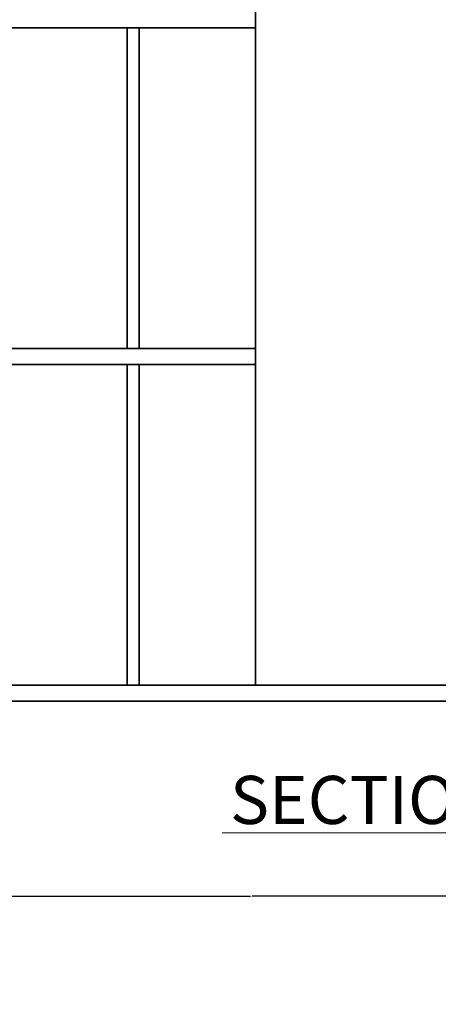
# Model space of a CAD drawing. Units: inches. Extents: x 2120 to 4013, y 1390 to 3019.
# Tile 57 of 59: x 3358 to 3515, y 2356 to 2724. Entities that reach past the tile are written whole.
import ezdxf

# ---------------------------------------------------------------- set-up
doc = ezdxf.new("R2010")
doc.units = ezdxf.units.IN
for name, color, linetype, lineweight in [('A-ANNO-DIMS', 2, 'Continuous', 18), ('A-ANNO-TEXT', 7, 'Continuous', 18), ('A-SECT', 7, 'Continuous', 35), ('A-WALL-PATT', 252, 'Continuous', 13)]:
    doc.layers.add(name, color=color, linetype=linetype, lineweight=lineweight)
doc.styles.get("Standard").update_dxf_attribs({"font": 'arial.ttf'})
doc.dimstyles.get("Standard").update_dxf_attribs({"dimtxt": 0.18, "dimasz": 0.18, "dimexe": 0.18, "dimexo": 0.0625, "dimgap": 0.09, "dimtad": 0, "dimtih": 1, "dimtoh": 1, "dimdec": 4, "dimzin": 0, "dimdsep": 46, "dimtxsty": 'Standard', "dimcen": 0.09, "dimadec": 0, "dimazin": 0, "dimtfac": 1, "dimtdec": 4, "dimtofl": 0, "dimtmove": 0, "dimatfit": 3, "dimfxl": 1, "dimtolj": 1, "dimtzin": 0, "dimarcsym": 0})

# ---------------------------------------------------------------- blocks, each defined once
blk = doc.blocks.new('*D216')
at = {"layer": 'A-ANNO-DIMS', "color": 0, "lineweight": -2, "transparency": 16777216}
for p, q in [((3071.73, 2352.59), (3071.73, 2396.46)), ((3071.91, 2396.28), (3444.95, 2396.28)), ((3818.55, 2396.28), (3445.52, 2396.28)), ((3818.73, 2352.59), (3818.73, 2396.46))]:
    blk.add_line(p, q, dxfattribs=at)
at = {"layer": 'A-ANNO-DIMS', "color": 0, "transparency": 16777216}
for points in [[(3071.91, 2396.31), (3071.91, 2396.25), (3071.73, 2396.28)], [(3818.55, 2396.31), (3818.55, 2396.25), (3818.73, 2396.28)]]:
    blk.add_solid(points, dxfattribs=at)
at = {"layer": 'Defpoints', "color": 0, "transparency": 16777216}
for p in [(3818.73, 2396.28), (3071.73, 2352.53), (3818.73, 2352.53)]:
    blk.add_point(p, dxfattribs=at)
at = {"layer": 'A-ANNO-DIMS', "color": 0, "transparency": 16777216, "insert": (3445.23, 2396.28), "char_height": 0.18, "attachment_point": 5}
blk.add_mtext('\\A1;747', dxfattribs=at)

msp = doc.modelspace()

# ---------------------------------------------------------------- hatches: boundary and pattern name
at = {"layer": 'A-WALL-PATT'}
h = msp.add_hatch(dxfattribs=at)
h.set_pattern_fill('ANSI32', color=256)
h.paths.add_polyline_path([(2271.7331, 2343.531), (2283.3788, 2343.531), (2283.3788, 2348.031), (2283.3788, 2352.5306), (2262.7331, 2352.5306), (2262.7331, 2182.638), (2267.2331, 2182.638), (2271.7331, 2182.638), (2271.7331, 2219.031), (2391.7331, 2219.031), (2391.7331, 2214.189), (2393.9831, 2214.189), (2396.2331, 2214.189), (2396.2331, 2219.031), (2420.2331, 2219.031), (2420.2331, 2225.7535), (2417.2197, 2225.7535), (2415.7331, 2225.7535), (2415.7331, 2223.5306), (2271.7331, 2223.5306)])
h.paths.add_polyline_path([(2380.0942, 2352.5306), (2343.3788, 2352.5306), (2343.3788, 2343.531), (2363.2331, 2343.531), (2363.2331, 2288.8489), (2365.4831, 2288.8489), (2367.7331, 2288.8489), (2367.7331, 2343.531), (2380.0942, 2343.531)], flags=17)
h.paths.add_polyline_path([(2432.4339, 2352.5306), (2404.0943, 2352.5306), (2404.0943, 2343.531), (2415.7331, 2343.531), (2415.7331, 2264.0306), (2367.7331, 2264.0306), (2367.7331, 2266.4872), (2363.2331, 2266.4872), (2363.2331, 2259.531), (2367.7331, 2259.531), (2415.7331, 2259.531), (2415.7331, 2255.0658), (2420.2331, 2255.0658), (2420.2331, 2259.531), (2424.5717, 2259.531), (2424.5717, 2261.781), (2424.5717, 2264.0306), (2420.2331, 2264.0306), (2420.2331, 2343.531), (2432.4339, 2343.531)])
h.paths.add_polyline_path([(2508.9115, 2352.5306), (2456.4339, 2352.5306), (2456.4339, 2343.531), (2468.2331, 2343.531), (2468.2331, 2264.0306), (2448.0487, 2264.0306), (2448.0487, 2259.531), (2468.2331, 2259.531), (2468.2331, 2255.5496), (2472.7331, 2255.5496), (2472.7331, 2343.531), (2508.9115, 2343.531)])
h.paths.add_polyline_path([(2637.7331, 2352.5306), (2544.9116, 2352.5306), (2544.9116, 2343.531), (2589.7331, 2343.531), (2633.2331, 2343.531), (2637.7331, 2343.531)])
h.paths.add_polyline_path([(2594.2331, 2343.5306), (2589.7331, 2343.5306), (2589.7331, 2259.5306), (2589.7331, 2252.4915), (2591.9831, 2252.4915), (2594.2331, 2252.4915)])
h.paths.add_polyline_path([(2637.7331, 2223.5306), (2594.2331, 2223.5306), (2594.2331, 2230.1988), (2591.9831, 2230.1988), (2589.7331, 2230.1988), (2589.7331, 2223.5306), (2472.7331, 2223.5306), (2468.2331, 2223.5306), (2468.2331, 2219.031), (2628.7331, 2219.031), (2628.7331, 2138.031), (2637.7331, 2138.031)])
h.paths.add_polyline_path([(3822.6535, 2458.4402), (3874.9468, 2458.4402), (3874.9468, 2476.9866), (3822.6535, 2476.9866)], flags=9)
h.paths.add_polyline_path([(3834.6921, 2781.8174), (3935.9206, 2781.8174), (3935.9206, 2800.3638), (3834.6921, 2800.3638)], flags=9)
h.paths.add_polyline_path([(3832.2843, 2837.9683), (3884.5776, 2837.9683), (3884.5776, 2856.5146), (3832.2843, 2856.5146)], flags=9)
h.paths.add_polyline_path([(3830.9388, 2861.4782), (3956.8958, 2861.4782), (3956.8958, 2880.0245), (3830.9388, 2880.0245)], flags=9)
h.paths.add_polyline_path([(3870.6966, 2352.5752), (3887.9272, 2352.5752), (3887.9272, 2377.3037), (3870.6966, 2377.3037)], flags=9)
h.paths.add_polyline_path([(3289.2701, 2413.161), (3435.2223, 2413.161), (3435.2223, 2450.2538), (3289.2701, 2450.2538)], flags=9)
h.paths.add_polyline_path([(2487.6944, 2414.3601), (2637.8335, 2414.3601), (2637.8335, 2451.4528), (2487.6944, 2451.4528)], flags=9)
h.paths.add_polyline_path([(2567.3724, 1457.9199), (2815.296, 1457.9199), (2815.296, 1495.0127), (2567.3724, 1495.0127)], flags=9)
h.paths.add_polyline_path([(2655.3825, 2093.2363), (2685.9555, 2093.2363), (2685.9555, 2111.8937), (2655.3825, 2111.8937)], flags=9)
h.paths.add_polyline_path([(2543.9218, 1550.6671), (2587.8406, 1550.6671), (2587.8406, 1569.3244), (2543.9218, 1569.3244)], flags=9)
h.paths.add_polyline_path([(2905.1384, 1543.8113), (2949.0572, 1543.8113), (2949.0572, 1562.4686), (2905.1384, 1562.4686)], flags=9)
h.paths.add_polyline_path([(2736.4118, 1702.4736), (2784.2153, 1702.4736), (2784.2153, 1721.1309), (2736.4118, 1721.1309)], flags=9)
h.paths.add_polyline_path([(2912.8666, 1710.4168), (2951.707, 1710.4168), (2951.707, 1729.0741), (2912.8666, 1729.0741)], flags=9)
h.paths.add_polyline_path([(2923.5785, 1763.5038), (2959.7279, 1763.5038), (2959.7279, 1782.1611), (2923.5785, 1782.1611)], flags=9)
h.paths.add_polyline_path([(2925.2114, 1809.6137), (2967.1861, 1809.6137), (2967.1861, 1828.271), (2925.2114, 1828.271)], flags=9)
h.paths.add_polyline_path([(2996.2711, 1878.9003), (2996.2711, 1913.109), (2977.6138, 1913.109), (2977.6138, 1878.9003)], flags=9)
h.paths.add_polyline_path([(2883.0859, 1895.7192), (2927.1855, 1895.7192), (2927.1855, 1914.3766), (2883.0859, 1914.3766)], flags=9)
h.paths.add_polyline_path([(2787.3924, 1810.8013), (2841.0213, 1810.8013), (2841.0213, 1829.4587), (2787.3924, 1829.4587)], flags=9)
h.paths.add_polyline_path([(2775.6399, 2101.7395), (2829.2689, 2101.7395), (2829.2689, 2120.3968), (2775.6399, 2120.3968)], flags=9)
h.paths.add_polyline_path([(2913.0263, 2075.817), (2951.8667, 2075.817), (2951.8667, 2094.4744), (2913.0263, 2094.4744)], flags=9)
h.paths.add_polyline_path([(2929.966, 2133.3669), (2966.1154, 2133.3669), (2966.1154, 2152.0243), (2929.966, 2152.0243)], flags=9)
h.paths.add_polyline_path([(2932.7502, 2182.6088), (2968.8996, 2182.6088), (2968.8996, 2201.2662), (2932.7502, 2201.2662)], flags=9)
h.paths.add_polyline_path([(2996.0681, 2266.3173), (2996.0681, 2300.5261), (2977.4108, 2300.5261), (2977.4108, 2266.3173)], flags=9)
h.paths.add_polyline_path([(2885.1039, 2279.2186), (2929.2035, 2279.2186), (2929.2035, 2297.8759), (2885.1039, 2297.8759)], flags=9)
h.paths.add_polyline_path([(2735.7042, 2218.3197), (2783.5078, 2218.3197), (2783.5078, 2236.9771), (2735.7042, 2236.9771)], flags=9)
h.paths.add_polyline_path([(2635.6049, 2044.0085), (2648.9678, 2044.0085), (2648.9678, 2054.312), (2635.6049, 2054.312)], flags=9)
h.paths.add_polyline_path([(2714.0148, 1923.0473), (2727.3777, 1923.0473), (2727.3777, 1933.3508), (2714.0148, 1933.3508)], flags=9)
h.paths.add_polyline_path([(2709.0345, 1988.1628), (2722.3974, 1988.1628), (2722.3974, 1998.4663), (2709.0345, 1998.4663)], flags=9)
h.paths.add_polyline_path([(2592.8935, 1962.1763), (2606.2564, 1962.1763), (2606.2564, 1972.4799), (2592.8935, 1972.4799)], flags=9)
h.paths.add_polyline_path([(2618.3996, 1985.9724), (2644.1942, 1985.9724), (2644.1942, 1996.2759), (2618.3996, 1996.2759)], flags=9)
h.paths.add_polyline_path([(2601.279, 1920.5869), (2614.6419, 1920.5869), (2614.6419, 1930.8904), (2601.279, 1930.8904)], flags=9)
h.paths.add_polyline_path([(2692.3278, 1932.7645), (2704.5311, 1932.7645), (2704.5311, 1943.0681), (2692.3278, 1943.0681)], flags=9)
h.paths.add_polyline_path([(2311.122, 1672.7318), (2355.0408, 1672.7318), (2355.0408, 1691.3892), (2311.122, 1691.3892)], flags=9)
h.paths.add_polyline_path([(2456.2551, 1632.3198), (2492.4796, 1632.3198), (2492.4796, 1650.9772), (2456.2551, 1650.9772)], flags=9)
h.paths.add_polyline_path([(2401.0766, 1631.4793), (2437.301, 1631.4793), (2437.301, 1650.1367), (2401.0766, 1650.1367)], flags=9)
h.paths.add_polyline_path([(2546.7054, 1700.9235), (2594.509, 1700.9235), (2594.509, 1719.5809), (2546.7054, 1719.5809)], flags=9)
h.paths.add_polyline_path([(2445.4866, 1766.9937), (2497.5261, 1766.9937), (2497.5261, 1785.651), (2445.4866, 1785.651)], flags=9)
h.paths.add_polyline_path([(2287.9992, 1739.7675), (2326.8396, 1739.7675), (2326.8396, 1758.4248), (2287.9992, 1758.4248)], flags=9)
h.paths.add_polyline_path([(2458.5279, 1924.7607), (2510.5675, 1924.7607), (2510.5675, 1943.4181), (2458.5279, 1943.4181)], flags=9)
h.paths.add_polyline_path([(2309.2811, 1902.7642), (2345.4305, 1902.7642), (2345.4305, 1921.4215), (2309.2811, 1921.4215)], flags=9)
h.paths.add_polyline_path([(2490.7554, 2018.9392), (2530.7896, 2018.9392), (2530.7896, 2037.5965), (2490.7554, 2037.5965)], flags=9)
h.paths.add_polyline_path([(2402.143, 2024.7393), (2438.5414, 2024.7393), (2438.5414, 2043.3966), (2402.143, 2043.3966)], flags=9)
h.paths.add_polyline_path([(2287.856, 1931.7926), (2326.6964, 1931.7926), (2326.6964, 1950.4499), (2287.856, 1950.4499)], flags=9)
h.paths.add_polyline_path([(2281.7979, 2193.5771), (2320.6383, 2193.5771), (2320.6383, 2212.2344), (2281.7979, 2212.2344)], flags=25)
h.paths.add_polyline_path([(2484.0754, 2093.892), (2536.115, 2093.892), (2536.115, 2112.5494), (2484.0754, 2112.5494)], flags=9)
h.paths.add_polyline_path([(2624.7948, 2281.8639), (2624.7948, 2311.4137), (2606.1375, 2311.4137), (2606.1375, 2281.8639)], flags=9)
h.paths.add_polyline_path([(2507.5036, 2290.3639), (2541.934, 2290.3639), (2541.934, 2309.0212), (2507.5036, 2309.0212)], flags=9)
h.paths.add_polyline_path([(2423.1076, 2285.2202), (2459.332, 2285.2202), (2459.332, 2303.8776), (2423.1076, 2303.8776)], flags=9)
h.paths.add_polyline_path([(2374.5467, 2289.6272), (2410.7711, 2289.6272), (2410.7711, 2308.2846), (2374.5467, 2308.2846)], flags=25)
h.paths.add_polyline_path([(2277.4907, 2227.5651), (2316.3311, 2227.5651), (2316.3311, 2246.2224), (2277.4907, 2246.2224)], flags=25)
h.paths.add_polyline_path([(2655.3825, 2093.2367), (2685.9555, 2093.2367), (2685.9555, 2111.894), (2655.3825, 2111.894)], flags=9)
h.paths.add_polyline_path([(2543.9217, 1550.6674), (2587.8406, 1550.6674), (2587.8406, 1569.3247), (2543.9217, 1569.3247)], flags=9)
h.paths.add_polyline_path([(2905.1384, 1543.8116), (2949.0572, 1543.8116), (2949.0572, 1562.4689), (2905.1384, 1562.4689)], flags=9)
h.paths.add_polyline_path([(2736.4118, 1702.4739), (2784.2153, 1702.4739), (2784.2153, 1721.1312), (2736.4118, 1721.1312)], flags=9)
h.paths.add_polyline_path([(2912.8666, 1710.4171), (2951.707, 1710.4171), (2951.707, 1729.0744), (2912.8666, 1729.0744)], flags=9)
h.paths.add_polyline_path([(2923.5785, 1763.5041), (2959.7279, 1763.5041), (2959.7279, 1782.1614), (2923.5785, 1782.1614)], flags=9)
h.paths.add_polyline_path([(2925.2114, 1809.614), (2967.1861, 1809.614), (2967.1861, 1828.2713), (2925.2114, 1828.2713)], flags=9)
h.paths.add_polyline_path([(2996.2711, 1878.9006), (2996.2711, 1913.1094), (2977.6137, 1913.1094), (2977.6137, 1878.9006)], flags=9)
h.paths.add_polyline_path([(2883.0859, 1895.7195), (2927.1855, 1895.7195), (2927.1855, 1914.3769), (2883.0859, 1914.3769)], flags=9)
h.paths.add_polyline_path([(2787.3924, 1810.8016), (2841.0213, 1810.8016), (2841.0213, 1829.459), (2787.3924, 1829.459)], flags=9)
h.paths.add_polyline_path([(2775.6399, 2101.7398), (2829.2688, 2101.7398), (2829.2688, 2120.3971), (2775.6399, 2120.3971)], flags=9)
h.paths.add_polyline_path([(2913.0263, 2075.8173), (2951.8667, 2075.8173), (2951.8667, 2094.4747), (2913.0263, 2094.4747)], flags=9)
h.paths.add_polyline_path([(2929.966, 2133.3672), (2966.1154, 2133.3672), (2966.1154, 2152.0246), (2929.966, 2152.0246)], flags=9)
h.paths.add_polyline_path([(2932.7502, 2182.6091), (2968.8996, 2182.6091), (2968.8996, 2201.2665), (2932.7502, 2201.2665)], flags=9)
h.paths.add_polyline_path([(2996.0681, 2266.3176), (2996.0681, 2300.5264), (2977.4108, 2300.5264), (2977.4108, 2266.3176)], flags=9)
h.paths.add_polyline_path([(2885.1039, 2279.2189), (2929.2035, 2279.2189), (2929.2035, 2297.8762), (2885.1039, 2297.8762)], flags=9)
h.paths.add_polyline_path([(2735.7042, 2218.32), (2783.5078, 2218.32), (2783.5078, 2236.9774), (2735.7042, 2236.9774)], flags=9)
h.paths.add_polyline_path([(2635.6048, 2044.0088), (2648.9677, 2044.0088), (2648.9677, 2054.3123), (2635.6048, 2054.3123)], flags=9)
h.paths.add_polyline_path([(2714.0148, 1923.0476), (2727.3777, 1923.0476), (2727.3777, 1933.3511), (2714.0148, 1933.3511)], flags=9)
h.paths.add_polyline_path([(2709.0345, 1988.1631), (2722.3974, 1988.1631), (2722.3974, 1998.4666), (2709.0345, 1998.4666)], flags=9)
h.paths.add_polyline_path([(2592.8935, 1962.1766), (2606.2564, 1962.1766), (2606.2564, 1972.4802), (2592.8935, 1972.4802)], flags=9)
h.paths.add_polyline_path([(2618.3995, 1985.9727), (2644.1942, 1985.9727), (2644.1942, 1996.2762), (2618.3995, 1996.2762)], flags=9)
h.paths.add_polyline_path([(2601.279, 1920.5872), (2614.6419, 1920.5872), (2614.6419, 1930.8908), (2601.279, 1930.8908)], flags=9)
h.paths.add_polyline_path([(2692.3278, 1932.7648), (2704.5311, 1932.7648), (2704.5311, 1943.0684), (2692.3278, 1943.0684)], flags=9)
h.paths.add_polyline_path([(2311.122, 1672.7321), (2355.0408, 1672.7321), (2355.0408, 1691.3895), (2311.122, 1691.3895)], flags=9)
h.paths.add_polyline_path([(2456.2551, 1632.3201), (2492.4795, 1632.3201), (2492.4795, 1650.9775), (2456.2551, 1650.9775)], flags=9)
h.paths.add_polyline_path([(2401.0766, 1631.4796), (2437.301, 1631.4796), (2437.301, 1650.137), (2401.0766, 1650.137)], flags=9)
h.paths.add_polyline_path([(2546.7054, 1700.9238), (2594.509, 1700.9238), (2594.509, 1719.5812), (2546.7054, 1719.5812)], flags=9)
h.paths.add_polyline_path([(2445.4866, 1766.994), (2497.5261, 1766.994), (2497.5261, 1785.6513), (2445.4866, 1785.6513)], flags=9)
h.paths.add_polyline_path([(2287.9992, 1739.7678), (2326.8396, 1739.7678), (2326.8396, 1758.4251), (2287.9992, 1758.4251)], flags=9)
h.paths.add_polyline_path([(2458.5279, 1924.7611), (2510.5675, 1924.7611), (2510.5675, 1943.4184), (2458.5279, 1943.4184)], flags=9)
h.paths.add_polyline_path([(2309.2811, 1902.7645), (2345.4305, 1902.7645), (2345.4305, 1921.4218), (2309.2811, 1921.4218)], flags=9)
h.paths.add_polyline_path([(2490.7554, 2018.9395), (2530.7895, 2018.9395), (2530.7895, 2037.5968), (2490.7554, 2037.5968)], flags=9)
h.paths.add_polyline_path([(2402.143, 2024.7396), (2438.5413, 2024.7396), (2438.5413, 2043.3969), (2402.143, 2043.3969)], flags=9)
h.paths.add_polyline_path([(2287.856, 1931.7929), (2326.6964, 1931.7929), (2326.6964, 1950.4502), (2287.856, 1950.4502)], flags=9)
h.paths.add_polyline_path([(2281.7979, 2193.5774), (2320.6383, 2193.5774), (2320.6383, 2212.2347), (2281.7979, 2212.2347)], flags=25)
h.paths.add_polyline_path([(2484.0754, 2093.8924), (2536.115, 2093.8924), (2536.115, 2112.5497), (2484.0754, 2112.5497)], flags=9)
h.paths.add_polyline_path([(2624.7948, 2281.8642), (2624.7948, 2311.414), (2606.1374, 2311.414), (2606.1374, 2281.8642)], flags=9)
h.paths.add_polyline_path([(2507.5035, 2290.3642), (2541.934, 2290.3642), (2541.934, 2309.0215), (2507.5035, 2309.0215)], flags=9)
h.paths.add_polyline_path([(2423.1075, 2285.2205), (2459.332, 2285.2205), (2459.332, 2303.8779), (2423.1075, 2303.8779)], flags=9)
h.paths.add_polyline_path([(2374.5467, 2289.6275), (2410.7711, 2289.6275), (2410.7711, 2308.2849), (2374.5467, 2308.2849)], flags=25)
h.paths.add_polyline_path([(2277.4907, 2227.5654), (2316.3311, 2227.5654), (2316.3311, 2246.2227), (2277.4907, 2246.2227)], flags=25)
h = msp.add_hatch(dxfattribs=at)
h.set_pattern_fill('ANSI32', color=256)
h.paths.add_polyline_path([(2271.7331, 1980.389), (2262.7331, 1980.389), (2262.7331, 1912.8434), (2267.2331, 1912.8434), (2271.7331, 1912.8434), (2271.7331, 1922.531), (2351.2331, 1922.531), (2351.2331, 1901.4728), (2355.7331, 1901.4728), (2355.7331, 1922.531), (2357.9815, 1922.531), (2357.9815, 1926.5306), (2271.7331, 1926.5306)])
h.paths.add_polyline_path([(2589.2331, 1949.1622), (2584.7331, 1949.1622), (2580.2331, 1949.1622), (2580.2331, 1874.5306), (2355.7331, 1874.5306), (2355.7331, 1880.1922), (2351.2331, 1880.1922), (2351.2331, 1874.5306), (2271.7331, 1874.5306), (2271.7331, 1888.8431), (2262.7331, 1888.8431), (2262.7331, 1842.2909), (2267.2331, 1842.2909), (2271.7331, 1842.2909), (2271.7331, 1865.531), (2415.7331, 1865.531), (2415.7331, 1779.7286), (2420.2331, 1779.7286), (2420.2331, 1865.531), (2589.2331, 1865.531)])
h.paths.add_polyline_path([(2271.7331, 1782.2906), (2262.7331, 1782.2906), (2262.7331, 1711.4639), (2267.2331, 1711.4639), (2271.7331, 1711.4639), (2271.7331, 1738.031), (2420.2331, 1738.031), (2420.2331, 1742.531), (2420.2331, 1747.3376), (2417.9831, 1747.3376), (2415.7331, 1747.3376), (2415.7331, 1742.5306), (2271.7331, 1742.5306)])
h.paths.add_polyline_path([(2271.7331, 1627.031), (2362.3957, 1627.031), (2362.3957, 1629.281), (2362.3957, 1631.5306), (2271.7331, 1631.5306), (2271.7331, 1675.4636), (2262.7331, 1675.4636), (2262.7331, 1581.531), (2405.3032, 1581.531), (2405.3032, 1586.031), (2405.3032, 1590.5306), (2396.2331, 1590.5306), (2396.2331, 1691.4513), (2418.7206, 1691.4513), (2418.7206, 1695.951), (2396.2331, 1695.951), (2391.7331, 1695.951), (2391.7331, 1631.5306), (2386.7425, 1631.5306), (2386.7425, 1629.2806), (2386.7425, 1627.031), (2391.7331, 1627.031), (2391.7331, 1586.1709), (2271.7331, 1586.1709)])
h.paths.add_polyline_path([(2459.6703, 1590.5306), (2429.3032, 1590.5306), (2429.3032, 1581.531), (2459.6703, 1581.531), (2459.6703, 1586.031)])
h.paths.add_polyline_path([(2501.2331, 1590.531), (2501.2331, 1665.0195), (2498.9831, 1665.0195), (2496.7331, 1665.0195), (2496.7331, 1590.5306), (2483.8201, 1590.5306), (2483.8201, 1590.1579), (2483.6704, 1590.1579), (2483.6704, 1581.531), (2505.0196, 1581.531), (2505.0196, 1583.781), (2505.0196, 1586.0306), (2501.2331, 1586.0306)])
h.paths.add_polyline_path([(2544.1361, 1583.781), (2544.1361, 1586.0306), (2527.1368, 1586.0306), (2527.1368, 1583.7806), (2527.1368, 1581.531), (2544.1361, 1581.531)])
h.paths.add_polyline_path([(3822.6535, 2458.4402), (3874.9468, 2458.4402), (3874.9468, 2476.9866), (3822.6535, 2476.9866)], flags=9)
h.paths.add_polyline_path([(3834.6921, 2781.8174), (3935.9206, 2781.8174), (3935.9206, 2800.3638), (3834.6921, 2800.3638)], flags=9)
h.paths.add_polyline_path([(3832.2843, 2837.9683), (3884.5776, 2837.9683), (3884.5776, 2856.5146), (3832.2843, 2856.5146)], flags=9)
h.paths.add_polyline_path([(3830.9388, 2861.4782), (3956.8958, 2861.4782), (3956.8958, 2880.0245), (3830.9388, 2880.0245)], flags=9)
h.paths.add_polyline_path([(3870.6966, 2352.5752), (3887.9272, 2352.5752), (3887.9272, 2377.3037), (3870.6966, 2377.3037)], flags=9)
h.paths.add_polyline_path([(3289.2701, 2413.161), (3435.2223, 2413.161), (3435.2223, 2450.2538), (3289.2701, 2450.2538)], flags=9)
h.paths.add_polyline_path([(2487.6944, 2414.3601), (2637.8335, 2414.3601), (2637.8335, 2451.4528), (2487.6944, 2451.4528)], flags=9)
h.paths.add_polyline_path([(2567.3724, 1457.9199), (2815.296, 1457.9199), (2815.296, 1495.0127), (2567.3724, 1495.0127)], flags=9)
h.paths.add_polyline_path([(2655.3825, 2093.2363), (2685.9555, 2093.2363), (2685.9555, 2111.8937), (2655.3825, 2111.8937)], flags=9)
h.paths.add_polyline_path([(2543.9218, 1550.6671), (2587.8406, 1550.6671), (2587.8406, 1569.3244), (2543.9218, 1569.3244)], flags=9)
h.paths.add_polyline_path([(2905.1384, 1543.8113), (2949.0572, 1543.8113), (2949.0572, 1562.4686), (2905.1384, 1562.4686)], flags=9)
h.paths.add_polyline_path([(2736.4118, 1702.4736), (2784.2153, 1702.4736), (2784.2153, 1721.1309), (2736.4118, 1721.1309)], flags=9)
h.paths.add_polyline_path([(2912.8666, 1710.4168), (2951.707, 1710.4168), (2951.707, 1729.0741), (2912.8666, 1729.0741)], flags=9)
h.paths.add_polyline_path([(2923.5785, 1763.5038), (2959.7279, 1763.5038), (2959.7279, 1782.1611), (2923.5785, 1782.1611)], flags=9)
h.paths.add_polyline_path([(2925.2114, 1809.6137), (2967.1861, 1809.6137), (2967.1861, 1828.271), (2925.2114, 1828.271)], flags=9)
h.paths.add_polyline_path([(2996.2711, 1878.9003), (2996.2711, 1913.109), (2977.6138, 1913.109), (2977.6138, 1878.9003)], flags=9)
h.paths.add_polyline_path([(2883.0859, 1895.7192), (2927.1855, 1895.7192), (2927.1855, 1914.3766), (2883.0859, 1914.3766)], flags=9)
h.paths.add_polyline_path([(2787.3924, 1810.8013), (2841.0213, 1810.8013), (2841.0213, 1829.4587), (2787.3924, 1829.4587)], flags=9)
h.paths.add_polyline_path([(2775.6399, 2101.7395), (2829.2689, 2101.7395), (2829.2689, 2120.3968), (2775.6399, 2120.3968)], flags=9)
h.paths.add_polyline_path([(2913.0263, 2075.817), (2951.8667, 2075.817), (2951.8667, 2094.4744), (2913.0263, 2094.4744)], flags=9)
h.paths.add_polyline_path([(2929.966, 2133.3669), (2966.1154, 2133.3669), (2966.1154, 2152.0243), (2929.966, 2152.0243)], flags=9)
h.paths.add_polyline_path([(2932.7502, 2182.6088), (2968.8996, 2182.6088), (2968.8996, 2201.2662), (2932.7502, 2201.2662)], flags=9)
h.paths.add_polyline_path([(2996.0681, 2266.3173), (2996.0681, 2300.5261), (2977.4108, 2300.5261), (2977.4108, 2266.3173)], flags=9)
h.paths.add_polyline_path([(2885.1039, 2279.2186), (2929.2035, 2279.2186), (2929.2035, 2297.8759), (2885.1039, 2297.8759)], flags=9)
h.paths.add_polyline_path([(2735.7042, 2218.3197), (2783.5078, 2218.3197), (2783.5078, 2236.9771), (2735.7042, 2236.9771)], flags=9)
h.paths.add_polyline_path([(2635.6049, 2044.0085), (2648.9678, 2044.0085), (2648.9678, 2054.312), (2635.6049, 2054.312)], flags=9)
h.paths.add_polyline_path([(2714.0148, 1923.0473), (2727.3777, 1923.0473), (2727.3777, 1933.3508), (2714.0148, 1933.3508)], flags=9)
h.paths.add_polyline_path([(2709.0345, 1988.1628), (2722.3974, 1988.1628), (2722.3974, 1998.4663), (2709.0345, 1998.4663)], flags=9)
h.paths.add_polyline_path([(2592.8935, 1962.1763), (2606.2564, 1962.1763), (2606.2564, 1972.4799), (2592.8935, 1972.4799)], flags=9)
h.paths.add_polyline_path([(2618.3996, 1985.9724), (2644.1942, 1985.9724), (2644.1942, 1996.2759), (2618.3996, 1996.2759)], flags=9)
h.paths.add_polyline_path([(2601.279, 1920.5869), (2614.6419, 1920.5869), (2614.6419, 1930.8904), (2601.279, 1930.8904)], flags=9)
h.paths.add_polyline_path([(2692.3278, 1932.7645), (2704.5311, 1932.7645), (2704.5311, 1943.0681), (2692.3278, 1943.0681)], flags=9)
h.paths.add_polyline_path([(2311.122, 1672.7318), (2355.0408, 1672.7318), (2355.0408, 1691.3892), (2311.122, 1691.3892)], flags=25)
h.paths.add_polyline_path([(2456.2551, 1632.3198), (2492.4796, 1632.3198), (2492.4796, 1650.9772), (2456.2551, 1650.9772)], flags=9)
h.paths.add_polyline_path([(2401.0766, 1631.4793), (2437.301, 1631.4793), (2437.301, 1650.1367), (2401.0766, 1650.1367)], flags=9)
h.paths.add_polyline_path([(2546.7054, 1700.9235), (2594.509, 1700.9235), (2594.509, 1719.5809), (2546.7054, 1719.5809)], flags=9)
h.paths.add_polyline_path([(2445.4866, 1766.9937), (2497.5261, 1766.9937), (2497.5261, 1785.651), (2445.4866, 1785.651)], flags=9)
h.paths.add_polyline_path([(2287.9992, 1739.7675), (2326.8396, 1739.7675), (2326.8396, 1758.4248), (2287.9992, 1758.4248)], flags=24)
h.paths.add_polyline_path([(2458.5279, 1924.7607), (2510.5675, 1924.7607), (2510.5675, 1943.4181), (2458.5279, 1943.4181)], flags=25)
h.paths.add_polyline_path([(2309.2811, 1902.7642), (2345.4305, 1902.7642), (2345.4305, 1921.4215), (2309.2811, 1921.4215)], flags=25)
h.paths.add_polyline_path([(2490.7554, 2018.9392), (2530.7896, 2018.9392), (2530.7896, 2037.5965), (2490.7554, 2037.5965)], flags=9)
h.paths.add_polyline_path([(2402.143, 2024.7393), (2438.5414, 2024.7393), (2438.5414, 2043.3966), (2402.143, 2043.3966)], flags=9)
h.paths.add_polyline_path([(2287.856, 1931.7926), (2326.6964, 1931.7926), (2326.6964, 1950.4499), (2287.856, 1950.4499)], flags=25)
h.paths.add_polyline_path([(2281.7979, 2193.5771), (2320.6383, 2193.5771), (2320.6383, 2212.2344), (2281.7979, 2212.2344)], flags=9)
h.paths.add_polyline_path([(2484.0754, 2093.892), (2536.115, 2093.892), (2536.115, 2112.5494), (2484.0754, 2112.5494)], flags=9)
h.paths.add_polyline_path([(2624.7948, 2281.8639), (2624.7948, 2311.4137), (2606.1375, 2311.4137), (2606.1375, 2281.8639)], flags=9)
h.paths.add_polyline_path([(2507.5036, 2290.3639), (2541.934, 2290.3639), (2541.934, 2309.0212), (2507.5036, 2309.0212)], flags=9)
h.paths.add_polyline_path([(2423.1076, 2285.2202), (2459.332, 2285.2202), (2459.332, 2303.8776), (2423.1076, 2303.8776)], flags=9)
h.paths.add_polyline_path([(2374.5467, 2289.6272), (2410.7711, 2289.6272), (2410.7711, 2308.2846), (2374.5467, 2308.2846)], flags=9)
h.paths.add_polyline_path([(2277.4907, 2227.5651), (2316.3311, 2227.5651), (2316.3311, 2246.2224), (2277.4907, 2246.2224)], flags=9)
h.paths.add_polyline_path([(2655.3825, 2093.2367), (2685.9555, 2093.2367), (2685.9555, 2111.894), (2655.3825, 2111.894)], flags=9)
h.paths.add_polyline_path([(2543.9217, 1550.6674), (2587.8406, 1550.6674), (2587.8406, 1569.3247), (2543.9217, 1569.3247)], flags=9)
h.paths.add_polyline_path([(2905.1384, 1543.8116), (2949.0572, 1543.8116), (2949.0572, 1562.4689), (2905.1384, 1562.4689)], flags=9)
h.paths.add_polyline_path([(2736.4118, 1702.4739), (2784.2153, 1702.4739), (2784.2153, 1721.1312), (2736.4118, 1721.1312)], flags=9)
h.paths.add_polyline_path([(2912.8666, 1710.4171), (2951.707, 1710.4171), (2951.707, 1729.0744), (2912.8666, 1729.0744)], flags=9)
h.paths.add_polyline_path([(2923.5785, 1763.5041), (2959.7279, 1763.5041), (2959.7279, 1782.1614), (2923.5785, 1782.1614)], flags=9)
h.paths.add_polyline_path([(2925.2114, 1809.614), (2967.1861, 1809.614), (2967.1861, 1828.2713), (2925.2114, 1828.2713)], flags=9)
h.paths.add_polyline_path([(2996.2711, 1878.9006), (2996.2711, 1913.1094), (2977.6137, 1913.1094), (2977.6137, 1878.9006)], flags=9)
h.paths.add_polyline_path([(2883.0859, 1895.7195), (2927.1855, 1895.7195), (2927.1855, 1914.3769), (2883.0859, 1914.3769)], flags=9)
h.paths.add_polyline_path([(2787.3924, 1810.8016), (2841.0213, 1810.8016), (2841.0213, 1829.459), (2787.3924, 1829.459)], flags=9)
h.paths.add_polyline_path([(2775.6399, 2101.7398), (2829.2688, 2101.7398), (2829.2688, 2120.3971), (2775.6399, 2120.3971)], flags=9)
h.paths.add_polyline_path([(2913.0263, 2075.8173), (2951.8667, 2075.8173), (2951.8667, 2094.4747), (2913.0263, 2094.4747)], flags=9)
h.paths.add_polyline_path([(2929.966, 2133.3672), (2966.1154, 2133.3672), (2966.1154, 2152.0246), (2929.966, 2152.0246)], flags=9)
h.paths.add_polyline_path([(2932.7502, 2182.6091), (2968.8996, 2182.6091), (2968.8996, 2201.2665), (2932.7502, 2201.2665)], flags=9)
h.paths.add_polyline_path([(2996.0681, 2266.3176), (2996.0681, 2300.5264), (2977.4108, 2300.5264), (2977.4108, 2266.3176)], flags=9)
h.paths.add_polyline_path([(2885.1039, 2279.2189), (2929.2035, 2279.2189), (2929.2035, 2297.8762), (2885.1039, 2297.8762)], flags=9)
h.paths.add_polyline_path([(2735.7042, 2218.32), (2783.5078, 2218.32), (2783.5078, 2236.9774), (2735.7042, 2236.9774)], flags=9)
h.paths.add_polyline_path([(2635.6048, 2044.0088), (2648.9677, 2044.0088), (2648.9677, 2054.3123), (2635.6048, 2054.3123)], flags=9)
h.paths.add_polyline_path([(2714.0148, 1923.0476), (2727.3777, 1923.0476), (2727.3777, 1933.3511), (2714.0148, 1933.3511)], flags=9)
h.paths.add_polyline_path([(2709.0345, 1988.1631), (2722.3974, 1988.1631), (2722.3974, 1998.4666), (2709.0345, 1998.4666)], flags=9)
h.paths.add_polyline_path([(2592.8935, 1962.1766), (2606.2564, 1962.1766), (2606.2564, 1972.4802), (2592.8935, 1972.4802)], flags=9)
h.paths.add_polyline_path([(2618.3995, 1985.9727), (2644.1942, 1985.9727), (2644.1942, 1996.2762), (2618.3995, 1996.2762)], flags=9)
h.paths.add_polyline_path([(2601.279, 1920.5872), (2614.6419, 1920.5872), (2614.6419, 1930.8908), (2601.279, 1930.8908)], flags=9)
h.paths.add_polyline_path([(2692.3278, 1932.7648), (2704.5311, 1932.7648), (2704.5311, 1943.0684), (2692.3278, 1943.0684)], flags=9)
h.paths.add_polyline_path([(2311.122, 1672.7321), (2355.0408, 1672.7321), (2355.0408, 1691.3895), (2311.122, 1691.3895)], flags=25)
h.paths.add_polyline_path([(2456.2551, 1632.3201), (2492.4795, 1632.3201), (2492.4795, 1650.9775), (2456.2551, 1650.9775)], flags=9)
h.paths.add_polyline_path([(2401.0766, 1631.4796), (2437.301, 1631.4796), (2437.301, 1650.137), (2401.0766, 1650.137)], flags=9)
h.paths.add_polyline_path([(2546.7054, 1700.9238), (2594.509, 1700.9238), (2594.509, 1719.5812), (2546.7054, 1719.5812)], flags=9)
h.paths.add_polyline_path([(2445.4866, 1766.994), (2497.5261, 1766.994), (2497.5261, 1785.6513), (2445.4866, 1785.6513)], flags=9)
h.paths.add_polyline_path([(2287.9992, 1739.7678), (2326.8396, 1739.7678), (2326.8396, 1758.4251), (2287.9992, 1758.4251)], flags=24)
h.paths.add_polyline_path([(2458.5279, 1924.7611), (2510.5675, 1924.7611), (2510.5675, 1943.4184), (2458.5279, 1943.4184)], flags=25)
h.paths.add_polyline_path([(2309.2811, 1902.7645), (2345.4305, 1902.7645), (2345.4305, 1921.4218), (2309.2811, 1921.4218)], flags=25)
h.paths.add_polyline_path([(2490.7554, 2018.9395), (2530.7895, 2018.9395), (2530.7895, 2037.5968), (2490.7554, 2037.5968)], flags=9)
h.paths.add_polyline_path([(2402.143, 2024.7396), (2438.5413, 2024.7396), (2438.5413, 2043.3969), (2402.143, 2043.3969)], flags=9)
h.paths.add_polyline_path([(2287.856, 1931.7929), (2326.6964, 1931.7929), (2326.6964, 1950.4502), (2287.856, 1950.4502)], flags=25)
h.paths.add_polyline_path([(2281.7979, 2193.5774), (2320.6383, 2193.5774), (2320.6383, 2212.2347), (2281.7979, 2212.2347)], flags=9)
h.paths.add_polyline_path([(2484.0754, 2093.8924), (2536.115, 2093.8924), (2536.115, 2112.5497), (2484.0754, 2112.5497)], flags=9)
h.paths.add_polyline_path([(2624.7948, 2281.8642), (2624.7948, 2311.414), (2606.1374, 2311.414), (2606.1374, 2281.8642)], flags=9)
h.paths.add_polyline_path([(2507.5035, 2290.3642), (2541.934, 2290.3642), (2541.934, 2309.0215), (2507.5035, 2309.0215)], flags=9)
h.paths.add_polyline_path([(2423.1075, 2285.2205), (2459.332, 2285.2205), (2459.332, 2303.8779), (2423.1075, 2303.8779)], flags=9)
h.paths.add_polyline_path([(2374.5467, 2289.6275), (2410.7711, 2289.6275), (2410.7711, 2308.2849), (2374.5467, 2308.2849)], flags=9)
h.paths.add_polyline_path([(2277.4907, 2227.5654), (2316.3311, 2227.5654), (2316.3311, 2246.2227), (2277.4907, 2246.2227)], flags=9)

# ---------------------------------------------------------------- linework, layer by layer
at = {"layer": 'A-ANNO-TEXT'}
msp.add_line((3578.9077, 2420.0416), (3434.336, 2420.0416), dxfattribs=at)
at = {"layer": 'A-SECT'}
for p, q in [((3446.7347, 2727.3118), (3446.7347, 2595.3118)), ((3446.7347, 2721.3118), (3071.7347, 2721.3118)), ((3398.7347, 2721.3118), (3398.7347, 2601.3118)), ((3403.2347, 2721.3118), (3403.2347, 2601.3118)), ((3446.7347, 2601.3118), (3071.7347, 2601.3118)), ((3446.7347, 2601.3118), (3446.7347, 2475.3118)), ((3446.7347, 2595.3118), (3071.7347, 2595.3118)), ((3398.7347, 2595.3118), (3398.7347, 2475.3118)), ((3403.2347, 2595.3118), (3403.2347, 2475.3118)), ((3818.7347, 2475.3118), (3071.7347, 2475.3118)), ((3071.7347, 2469.3118), (3818.7347, 2469.3118))]:
    msp.add_line(p, q, dxfattribs=at)

# ---------------------------------------------------------------- texts
at = {"layer": 'A-ANNO-TEXT', "insert": (3437.2118, 2441.309), "char_height": 18, "attachment_point": 1}
msp.add_mtext_dynamic_manual_height_columns('SECTION-A', width=601.378558, gutter_width=12.5, heights=[0], dxfattribs=at)

# ---------------------------------------------------------------- dimensions: what is measured, and where the dimension line sits
at = {"layer": 'A-ANNO-DIMS'}
dim = msp.add_linear_dim(base=(3818.7347, 2396.281), p1=(3071.7347, 2352.531), p2=(3818.7347, 2352.531), dimstyle='Standard', override={"dimdec": 0, "dimlfac": 1, "dimrnd": 0, "dimzin": 0, "dimdsep": 46, "dimlunit": 2}, dxfattribs=at)
dim.commit()
dim.dimension.update_dxf_attribs({"geometry": '*D216', "text_midpoint": (3445.2347, 2396.281)})

doc.saveas('drawing.dxf')
